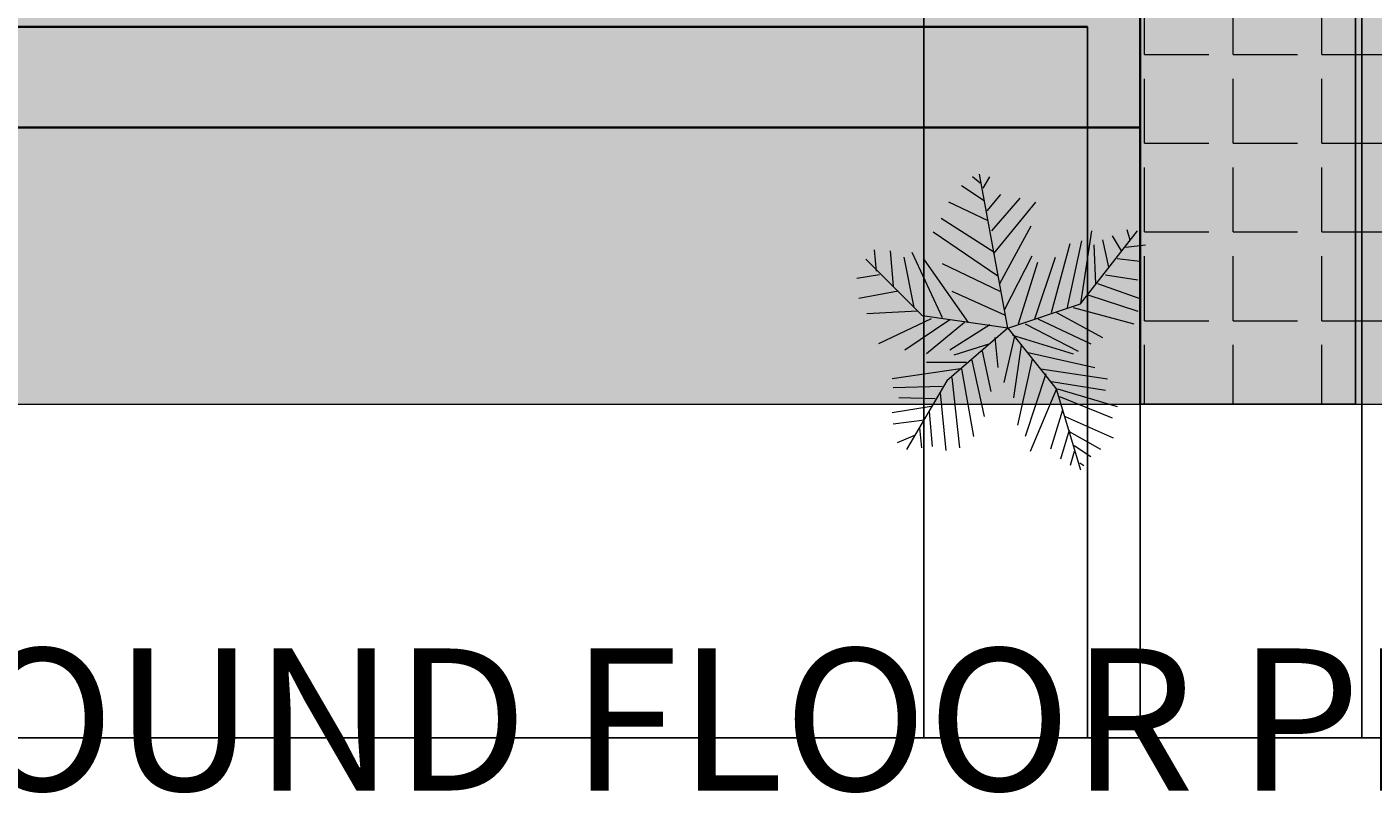
# Model space of a CAD drawing. Units: millimetres. Extents: x 1166 to 16630, y -7192 to 2820.
# Tile 2 of 8: x 2769 to 5842, y -7192 to -5443. Entities that reach past the tile are written whole.
import ezdxf

# ---------------------------------------------------------------- set-up
doc = ezdxf.new("R2010")
doc.units = ezdxf.units.MM
for name, color, linetype, lineweight in [('A-ANNO-DIMS', 2, 'Continuous', 18), ('A-ANNO-TEXT', 7, 'Continuous', 35), ('A-FLOR-PATT', 8, 'Continuous', 13), ('A-WALL', 7, 'Continuous', 35), ('C-SITE-PAVE', 7, 'Continuous', 18), ('L-PLNT', 70, 'Continuous', 18), ('L-PLNT-PATT', 3, 'Continuous', 13)]:
    doc.layers.add(name, color=color, linetype=linetype, lineweight=lineweight)
doc.layers.add('A-FLOR-FNSH-PATT', color=254, linetype='Continuous', lineweight=13, true_color=0xfeeab9)
doc.layers.add('A-WALL-PATT', color=254, linetype='Continuous', lineweight=13, true_color=0xcecce6)
doc.styles.get("Standard").update_dxf_attribs({"font": 'arial.ttf'})
doc.dimstyles.get("Standard").update_dxf_attribs({"dimtxt": 0.18, "dimasz": 0.18, "dimexe": 0.18, "dimexo": 0.0625, "dimgap": 0.09, "dimtad": 0, "dimtih": 1, "dimtoh": 1, "dimdec": 4, "dimzin": 0, "dimdsep": 46, "dimtxsty": 'Standard', "dimcen": 0.09, "dimadec": 0, "dimazin": 0, "dimtfac": 1, "dimtdec": 4, "dimtofl": 0, "dimtmove": 0, "dimatfit": 3, "dimfxl": 1, "dimtolj": 1, "dimtzin": 0, "dimarcsym": 0})

# ---------------------------------------------------------------- blocks, each defined once
blk = doc.blocks.new('*U12')
for p, q in [((-10.186, 53.64), (-13.084, 55.962)), ((0, 0), (-10.5, 57)), ((-9.099, 51.782), (-6.563, 55.962)), ((-8.737, 47.138), (-17.069, 52.711)), ((-7.288, 39.707), (-21.778, 46.673)), ((-7.65, 43.423), (-2.578, 49.46)), ((-5.839, 35.992), (4.667, 48.067)), ((-5.114, 27.632), (10.463, 46.673)), ((-5.114, 28.097), (-24.676, 40.636)), ((-3.665, 19.273), (-27.574, 35.527)), ((-2.941, 16.486), (8.652, 37.85)), ((27, 9), (48, 36)), ((27.127, 9.056), (31.112, 35.992)), ((44.153, 36.456), (45.239, 32.741)), ((16.259, 5.805), (23.142, 31.348)), ((22.055, 7.198), (27.489, 32.277)), ((31.836, 30.883), (32.561, 16.486)), ((35.096, 32.741), (37.27, 22.524)), ((38.719, 34.134), (41.979, 28.561)), ((43.791, 29.954), (51.036, 30.883)), ((-31.5, 4.5), (-52.5, 25.5)), ((-48.585, 21.131), (-49.309, 29.026)), ((-43.513, 28.561), (-42.427, 15.558)), ((-38.442, 26.239), (-34.819, 7.663)), ((-35.544, 28.097), (-24.314, 3.947)), ((-14.533, 2.09), (-30.834, 25.31)), ((-1.129, 6.734), (9.014, 26.704)), ((10.101, 3.483), (17.708, 26.239)), ((40.53, 25.775), (48.862, 24.846)), ((-24.314, 23.917), (-2.941, 13.7)), ((3.942, 1.625), (11.187, 24.381)), ((-47.498, 19.737), (-55.83, 18.344)), ((33.285, 16.486), (48.862, 10.913)), ((36.183, 19.737), (48.137, 17.88)), ((-40.615, 13.7), (-55.105, 10.913)), ((-20.691, 13.7), (-1.129, 4.876)), ((29.662, 12.307), (48.137, 6.269)), ((-33.37, 6.269), (-52.207, 5.34)), ((0, 0), (27, 9)), ((18.07, 5.805), (35.096, -3.483)), ((24.229, 7.663), (46.688, 1.625)), ((-28.299, 3.483), (-47.86, -5.805)), ((-21.416, 3.018), (-38.079, -8.128)), ((0, 0), (-31.5, 4.5)), ((-15.982, 2.09), (-30.11, -9.521)), ((0, 0), (-22.5, -19.5)), ((-6.563, 1.161), (-21.416, -8.128)), ((0, 0), (18, -22.5)), ((6.478, 1.625), (26.04, -8.592)), ((11.187, 3.483), (30.749, -5.805)), ((-4.752, -3.483), (-3.665, -14.629)), ((2.493, -3.019), (-1.491, -20.202)), ((1.769, -2.555), (24.229, -9.521)), ((-6.563, -5.805), (-19.967, -9.985)), ((-9.461, -8.592), (-6.201, -23.453)), ((5.029, -6.27), (2.131, -25.775)), ((7.565, -9.056), (32.198, -14.629)), ((-15.257, -12.772), (-30.11, -12.772)), ((-13.446, -11.378), (-8.737, -32.741)), ((9.014, -11.378), (3.58, -35.992)), ((-17.431, -15.094), (-42.789, -18.809)), ((-22.5, -19.5), (-37.5, -45)), ((-20.691, -18.345), (-17.793, -44.352)), ((-17.069, -15.094), (-12.721, -40.172)), ((14.085, -16.951), (6.478, -40.172)), ((12.274, -15.094), (36.907, -18.809)), ((16.259, -19.738), (36.183, -22.989)), ((-24.314, -21.596), (-42.427, -22.06)), ((-25.038, -23.918), (-22.865, -45.281)), ((18.07, -22.524), (8.289, -45.745)), ((18, -22.5), (27, -52.5)), ((18.433, -22.524), (40.53, -29.026)), ((-28.299, -29.026), (-42.789, -31.348)), ((-26.849, -26.24), (-40.253, -25.775)), ((19.157, -25.311), (38.719, -33.206)), ((-30.834, -34.135), (-42.427, -35.528)), ((-29.023, -30.884), (-27.936, -43.887)), ((20.244, -30.419), (15.897, -44.816)), ((21.331, -32.741), (39.081, -40.636)), ((-34.457, -39.708), (-40.978, -42.494)), ((-32.646, -36.921), (-31.921, -44.352)), ((22.78, -37.85), (19.519, -48.532)), ((22.78, -38.314), (34.372, -44.816)), ((24.591, -43.423), (30.749, -47.603)), ((24.591, -45.745), (23.142, -50.854)), ((26.764, -49.925), (28.213, -50.854))]:
    blk.add_line(p, q)
blk = doc.blocks.new('*D31')
at = {"layer": 'A-ANNO-DIMS', "color": 0, "lineweight": -2, "transparency": 16777216}
for p, q in [((1957, -5450.9), (1957, -7065.6)), ((5189.6, -5442.6), (5189.6, -7065.6)), ((1957.2, -7065.4), (3572.8, -7065.4)), ((5189.4, -7065.4), (3573.8, -7065.4))]:
    blk.add_line(p, q, dxfattribs=at)
at = {"layer": 'A-ANNO-DIMS', "color": 0, "transparency": 16777216}
for points in [[(1957.2, -7065.4), (1957.2, -7065.5), (1957, -7065.4)], [(5189.4, -7065.4), (5189.4, -7065.5), (5189.6, -7065.4)]]:
    blk.add_solid(points, dxfattribs=at)
at = {"layer": 'Defpoints', "color": 0, "transparency": 16777216}
for p in [(1957, -5450.8), (5189.6, -5442.5), (5189.6, -7065.4)]:
    blk.add_point(p, dxfattribs=at)
at = {"layer": 'A-ANNO-DIMS', "color": 0, "transparency": 16777216, "insert": (3573.3, -7065.4), "char_height": 0.18, "attachment_point": 5}
blk.add_mtext('\\A1;3232.6', dxfattribs=at)
blk = doc.blocks.new('*D32')
at = {"layer": 'A-ANNO-DIMS', "color": 0, "lineweight": -2, "transparency": 16777216}
for p, q in [((5309.6, -6304.2), (5309.6, -7065.6)), ((7725.9, -6304.2), (7725.9, -7065.6)), ((5309.8, -7065.4), (6517.3, -7065.4)), ((7725.8, -7065.4), (6518.2, -7065.4))]:
    blk.add_line(p, q, dxfattribs=at)
at = {"layer": 'A-ANNO-DIMS', "color": 0, "transparency": 16777216}
for points in [[(5309.8, -7065.4), (5309.8, -7065.5), (5309.6, -7065.4)], [(7725.8, -7065.4), (7725.8, -7065.5), (7725.9, -7065.4)]]:
    blk.add_solid(points, dxfattribs=at)
at = {"layer": 'Defpoints', "color": 0, "transparency": 16777216}
for p in [(5309.6, -6304.1), (7725.9, -6304.1), (7725.9, -7065.4)]:
    blk.add_point(p, dxfattribs=at)
at = {"layer": 'A-ANNO-DIMS', "color": 0, "transparency": 16777216, "insert": (6517.8, -7065.4), "char_height": 0.18, "attachment_point": 5}
blk.add_mtext('\\A1;2416.3', dxfattribs=at)
blk = doc.blocks.new('*D36')
at = {"layer": 'A-ANNO-DIMS', "color": 0, "lineweight": -2, "transparency": 16777216}
for p, q in [((4815.9, -849.9), (4815.9, -7065.6)), ((5815.9, -849.9), (5815.9, -7065.6)), ((4816.1, -7065.4), (5315.6, -7065.4)), ((5815.8, -7065.4), (5316.3, -7065.4))]:
    blk.add_line(p, q, dxfattribs=at)
at = {"layer": 'A-ANNO-DIMS', "color": 0, "transparency": 16777216}
for points in [[(4816.1, -7065.4), (4816.1, -7065.5), (4815.9, -7065.4)], [(5815.8, -7065.4), (5815.8, -7065.5), (5815.9, -7065.4)]]:
    blk.add_solid(points, dxfattribs=at)
at = {"layer": 'Defpoints', "color": 0, "transparency": 16777216}
for p in [(4815.9, -849.8), (5815.9, -849.8), (5815.9, -7065.4)]:
    blk.add_point(p, dxfattribs=at)
at = {"layer": 'A-ANNO-DIMS', "color": 0, "transparency": 16777216, "insert": (5315.9, -7065.4), "char_height": 0.18, "attachment_point": 5}
blk.add_mtext('\\A1;1000', dxfattribs=at)
blk = doc.blocks.new('*D39')
at = {"layer": 'A-ANNO-DIMS', "color": 0, "lineweight": -2, "transparency": 16777216}
for p, q in [((5309.7, -2642.5), (5801.8, -2642.5)), ((5801.6, -2642.7), (5801.6, -4473.2)), ((5801.6, -6304), (5801.6, -4473.5)), ((5309.7, -6304.1), (5801.8, -6304.1))]:
    blk.add_line(p, q, dxfattribs=at)
at = {"layer": 'A-ANNO-DIMS', "color": 0, "transparency": 16777216}
for points in [[(5801.6, -2642.7), (5801.6, -2642.7), (5801.6, -2642.5)], [(5801.6, -6304), (5801.6, -6304), (5801.6, -6304.1)]]:
    blk.add_solid(points, dxfattribs=at)
at = {"layer": 'Defpoints', "color": 0, "transparency": 16777216}
for p in [(5309.6, -2642.5), (5309.6, -6304.1), (5801.6, -6304.1)]:
    blk.add_point(p, dxfattribs=at)
at = {"layer": 'A-ANNO-DIMS', "color": 0, "transparency": 16777216, "insert": (5801.6, -4473.3), "char_height": 0.18, "attachment_point": 5}
blk.add_mtext('\\A1;3661.6', dxfattribs=at)

msp = doc.modelspace()

# ---------------------------------------------------------------- hatches: boundary and pattern name
at = {"layer": 'A-FLOR-FNSH-PATT', "transparency": 33554523}
h = msp.add_hatch(color=256, dxfattribs=at)
h.dxf.hatch_style = 1
h.paths.add_polyline_path([(7725.939, 2327.462), (1725.939, 2327.462), (1725.939, -5672.538), (5309.615, -5672.538), (5309.615, -2642.538), (5189.615, -2642.538), (5189.615, -5442.538), (1955.939, -5442.538), (1955.939, 2097.462), (4665.939, 2097.462), (4665.939, 150.2), (4815.939, 150.2, -0.40145271), (5814.982, -806.05), (5815.939, -806.05), (5815.939, -849.8), (4815.939, -849.8), (4785.939, -849.8), (4785.939, -902.538), (7495.939, -902.538), (7495.939, -2522.538), (4884.014, -2522.538), (4884.014, -2642.538), (7725.939, -2642.538)], flags=17)
h.paths.add_polyline_path([(6066.077, 618.421), (6066.077, 1624.186), (7407.098, 1624.186), (7407.098, 618.421)], flags=16)
h.paths.add_polyline_path([(4979.212, 660.219), (4799.278, 660.219), (4799.278, 780.174), (4789.282, 790.171), (4789.282, 870.141), (4799.278, 880.137), (4799.278, 1259.997), (4979.212, 1259.997), (4979.212, 1230.008), (4989.208, 1230.008), (4989.208, 1110.052), (4979.212, 1110.052), (4979.212, 1100.056), (4989.208, 1100.056), (4989.208, 980.1), (4979.212, 980.1), (4979.212, 950.111), (4989.208, 950.111), (4989.208, 940.115, -0.09090909), (4989.208, 720.196), (4989.208, 710.2), (4979.212, 710.2)], flags=16)
h.paths.add_polyline_path([(4974.214, 665.217), (4804.276, 665.217), (4804.276, 1254.999), (4974.214, 1254.999)], flags=0)
h.paths.add_polyline_path([(6910.92, 618.421), (6910.92, 873.215), (7165.714, 873.215), (7165.714, 1490.084), (7386.983, 1490.084), (7386.983, 1141.419), (7165.714, 1141.419), (7165.714, 1101.188), (7386.983, 1101.188), (7386.983, 752.523), (7132.189, 752.523), (7132.189, 839.689)], flags=16)
h.paths.add_polyline_path([(4815.939, 150.2), (4665.939, 150.2), (4665.939, 1500.697), (2460.545, 1500.697), (2460.545, -402.538), (3575.939, -402.538), (3575.939, -1706.64), (3463.439, -1706.64, 0.40145271), (2714.158, -2423.828), (3463.439, -2423.828), (3463.439, -2456.64), (3455.939, -2522.538), (3455.939, -2456.64), (2713.439, -2456.64), (2713.439, -2423.828), (2714.158, -2423.828, -0.39855266), (3455.939, -1706.678), (3455.939, -1706.64), (3575.939, -1706.64), (3575.939, -402.538), (2460.545, -402.538), (2460.545, 1500.697), (4665.939, 1500.697), (4665.939, 150.2), (4785.939, 150.2), (4785.939, 2097.462), (7495.939, 2097.462), (7495.939, -2522.538), (4884.014, -2522.538), (4884.014, -2642.538), (7725.939, -2642.538), (7725.939, 2327.462), (1725.939, 2327.462), (1725.939, -5672.538), (5309.615, -5672.538), (5309.615, -2642.538), (4884.014, -2642.538), (4884.014, -2522.538), (4884.014, -1822.538), (4665.939, -1822.538), (4665.939, -1722.538), (4665.939, -1022.538), (4665.939, -849.8), (4815.939, -849.8), (4815.939, -806.05), (5814.982, -806.05, 0.40145271)])
h.paths.add_polyline_path([(1955.939, -4323.626), (1965.936, -4313.63), (1965.936, -3933.77), (2145.869, -3933.77), (2145.869, -3963.759), (2155.866, -3963.759), (2155.866, -4083.715), (2145.869, -4083.715), (2145.869, -4093.711), (2155.866, -4093.711), (2155.866, -4213.667), (2145.869, -4213.667), (2145.869, -4243.656), (2155.866, -4243.656), (2155.866, -4253.652, -0.09090909), (2155.866, -4473.571), (2155.866, -4483.567), (2145.869, -4483.567), (2145.869, -4533.549), (1965.936, -4533.549), (1965.936, -4413.593), (1955.939, -4403.597)], flags=16)
h.paths.add_polyline_path([(3017.672, -1268.685), (3017.672, -1558.932), (2092.538, -1558.932), (2092.538, -1268.685)], flags=16)
h.paths.add_polyline_path([(2768.799, -687.028), (2664.904, -687.028), (2696.871, -782.93, -0.50132349), (2617.667, -1084.405, -0.13289091), (2584.271, -1084.405, -0.50131678), (2505.065, -782.933), (2537.033, -687.028), (2489.082, -687.028), (2489.082, -711.004), (2441.13, -711.004), (2441.13, -687.028), (2433.138, -687.028), (2433.138, -559.158), (2768.799, -559.158)], flags=16)
h.paths.add_polyline_path([(2752.815, -655.061, -0.41421356), (2740.827, -671.045), (2465.106, -671.045, -0.41421356), (2449.122, -659.057), (2449.122, -591.126, -0.41421356), (2461.11, -575.142), (2736.831, -575.142, -0.41421356), (2752.815, -587.13)], flags=0)
h.paths.add_polyline_path([(2627.247, -1063.016, -0.21500378), (2574.691, -1063.016, -0.48007965), (2537.034, -782.931), (2664.904, -782.931, -0.4800795)], flags=0)
h.paths.add_polyline_path([(4505.634, -3647.875), (4977.863, -3647.875, -0.19047621), (4977.864, -5173.541), (4505.634, -5173.541), (4505.634, -5064.565), (4533.929, -5064.565), (4533.929, -3756.851), (4505.634, -3756.851)], flags=16)
h.paths.add_polyline_path([(4880.114, -4192.756), (5003.372, -4192.756, -0.04962821), (5003.372, -4628.66), (4880.114, -4628.66)], flags=0)
h.paths.add_polyline_path([(2140.871, -3938.769), (2140.871, -4528.551), (1970.934, -4528.551), (1970.934, -3938.769)], flags=0)
h.paths.add_polyline_path([(7495.939, -1022.538), (6660.699, -1022.538), (6660.699, -1722.538, -0.21291191), (6697.901, -1739.132)], flags=16)
h.paths.add_polyline_path([(7495.939, -1022.538), (6697.901, -1739.132, -0.18498743), (6710.699, -1772.538), (7495.939, -1772.538)], flags=16)
h.paths.add_polyline_path([(7495.939, -1772.538), (6710.699, -1772.538, -0.18498743), (6697.901, -1805.944), (7495.939, -2522.538)], flags=16)
h.paths.add_polyline_path([(6697.901, -1805.944, -0.21291191), (6660.699, -1822.538), (6660.699, -2522.538), (7495.939, -2522.538)], flags=16)
h.paths.add_polyline_path([(6660.699, -1822.538), (6438.613, -1822.538), (6438.613, -2522.538), (6660.699, -2522.538)], flags=16)
h.paths.add_polyline_path([(6438.613, -1822.538), (6216.528, -1822.538), (6216.528, -2522.538), (6438.613, -2522.538)], flags=16)
h.paths.add_polyline_path([(6216.528, -1822.538), (5994.442, -1822.538), (5994.442, -2522.538), (6216.528, -2522.538)], flags=16)
h.paths.add_polyline_path([(5994.442, -1822.538), (5772.357, -1822.538), (5772.357, -2522.538), (5994.442, -2522.538)], flags=16)
h.paths.add_polyline_path([(5550.271, -1822.538), (5328.185, -1822.538), (5328.185, -2522.538), (5550.271, -2522.538)], flags=16)
h.paths.add_polyline_path([(5328.185, -1822.538), (5106.1, -1822.538), (5106.1, -2522.538), (5328.185, -2522.538)], flags=16)
h.paths.add_polyline_path([(5106.1, -1822.538), (4884.014, -1822.538), (4884.014, -2522.538), (5106.1, -2522.538)], flags=16)
h.paths.add_polyline_path([(4884.014, -1022.538), (4665.939, -1022.538), (4665.939, -1722.538), (4884.014, -1722.538)], flags=16)
h.paths.add_polyline_path([(5106.1, -1022.538), (4884.014, -1022.538), (4884.014, -1722.538), (5106.1, -1722.538)], flags=16)
h.paths.add_polyline_path([(5550.271, -1022.538), (5328.185, -1022.538), (5328.185, -1722.538), (5550.271, -1722.538)], flags=16)
h.paths.add_polyline_path([(5328.185, -1022.538), (5106.1, -1022.538), (5106.1, -1722.538), (5328.185, -1722.538)], flags=16)
h.paths.add_polyline_path([(5772.357, -1022.538), (5550.271, -1022.538), (5550.271, -1722.538), (5772.357, -1722.538)], flags=16)
h.paths.add_polyline_path([(5994.442, -1022.538), (5772.357, -1022.538), (5772.357, -1722.538), (5994.442, -1722.538)], flags=16)
h.paths.add_polyline_path([(6216.528, -1022.538), (5994.442, -1022.538), (5994.442, -1722.538), (6216.528, -1722.538)], flags=16)
h.paths.add_polyline_path([(6660.699, -1022.538), (6438.613, -1022.538), (6438.613, -1722.538), (6660.699, -1722.538)], flags=16)
h.paths.add_polyline_path([(6438.613, -1022.538), (6216.528, -1022.538), (6216.528, -1722.538), (6438.613, -1722.538)], flags=16)
h.paths.add_polyline_path([(5772.357, -1822.538), (5550.271, -1822.538), (5550.271, -2522.538), (5772.357, -2522.538)], flags=16)
h.paths.add_polyline_path([(6660.699, -1722.538), (6438.613, -1722.538), (4665.939, -1722.538), (4665.939, -1822.538), (6660.699, -1822.538, 0.21291191), (6697.901, -1805.944, 0.64892437)], flags=16)
h.paths.add_polyline_path([(5860.25, -44.006), (7154.504, -44.006), (7154.504, 215.689), (5860.25, 215.689)], flags=24)
h.paths.add_polyline_path([(2102.336, -1543.656), (3007.075, -1543.656), (3007.075, -1283.961), (2102.336, -1283.961)], flags=8)
h.paths.add_polyline_path([(2887.503, -4248.68), (3740.372, -4248.68), (3740.372, -3989.156), (2887.503, -3989.156)], flags=24)
h.paths.add_polyline_path([(2999.436, 433.054), (4111.829, 433.054), (4111.829, 692.578), (2999.436, 692.578)], flags=24)
at = {"layer": 'A-FLOR-FNSH-PATT', "transparency": 33554590}
h = msp.add_hatch(color=256, dxfattribs=at)
h.dxf.hatch_style = 1
h.paths.add_polyline_path([(5309.615, -2642.538), (5309.615, -6304.141), (7725.939, -6304.141), (7725.939, -5672.538), (7725.939, -2642.538)])
edge = h.paths.add_edge_path(flags=16)
edge.add_ellipse((-448.972, -3645.43), major_axis=(-7430.723, 0), ratio=0.84230387, start_angle=182.1799503, end_angle=183.6504276, ccw=False)
edge.add_line((6974.174, -3362.862), (6984.716, -3362.862))
edge.add_ellipse((6982.281, -3380.397), major_axis=(-20.817, 0), ratio=0.84230387, start_angle=180, end_angle=270, ccw=False)
edge.add_line((7003.098, -3380.397), (7003.098, -3722.916))
edge.add_ellipse((6982.281, -3720.865), major_axis=(20.817, 0), ratio=0.84230387, start_angle=270, end_angle=360, ccw=False)
edge.add_ellipse((-142030.923, -3973.064), major_axis=(149013.204, 0), ratio=0.8423038695, start_angle=-0.38386678, end_angle=0.09022909, ccw=False)
edge.add_line((6977.567, -4971.397), (6984.47, -4971.397))
edge.add_ellipse((6982.281, -4988.932), major_axis=(20.817, 0), ratio=0.84230387, start_angle=0, end_angle=90, ccw=False)
edge.add_line((7003.098, -4988.932), (7003.098, -5331.243))
edge.add_ellipse((6982.281, -5329.4), major_axis=(-20.817, 0), ratio=0.84230387, start_angle=90, end_angle=180, ccw=False)
edge.add_line((6982.281, -5346.934), (6973.354, -5346.934))
edge.add_ellipse((-142030.923, -3973.064), major_axis=(149013.204, 0), ratio=0.8423038695, start_angle=-0.6186432, end_angle=-0.52827147, ccw=False)
edge.add_ellipse((6960.189, -5606.903), major_axis=(-31.226, 0), ratio=0.84230387, start_angle=179.371763, end_angle=248.464757, ccw=False)
edge.add_ellipse((-142041.332, -3973.064), major_axis=(-149045.372, 0), ratio=0.8423038661, start_angle=179.35344592, end_angle=179.3717628, ccw=False)
edge.add_ellipse((6916.87, -5654.054), major_axis=(-73.802, 0), ratio=0.84230387, start_angle=90, end_angle=179.353446, ccw=False)
edge.add_line((6916.87, -5716.218), (5995.23, -5716.218))
edge.add_ellipse((5995.23, -5654.054), major_axis=(73.802, 0), ratio=0.84230387, start_angle=180.646554, end_angle=270, ccw=False)
edge.add_ellipse((154953.432, -3973.064), major_axis=(-149045.372, 0), ratio=0.8423038697, start_angle=0.62823722, end_angle=0.6465541, ccw=False)
edge.add_ellipse((5951.911, -5606.903), major_axis=(31.226, 0), ratio=0.84230387, start_angle=111.535244, end_angle=180.628237, ccw=False)
edge.add_ellipse((154943.023, -3973.064), major_axis=(-149013.204, 0), ratio=0.8423038695, start_angle=0.52827147, end_angle=0.6465541, ccw=False)
edge.add_line((5938.746, -5346.934), (5927.384, -5346.934))
edge.add_ellipse((5929.819, -5329.4), major_axis=(20.817, 0), ratio=0.84230387, start_angle=180, end_angle=270, ccw=False)
edge.add_line((5909.002, -5329.4), (5909.002, -4986.881))
edge.add_ellipse((5929.819, -4988.932), major_axis=(-20.817, 0), ratio=0.84230387, start_angle=-90, end_angle=0, ccw=False)
edge.add_line((5929.819, -4971.397), (5934.533, -4971.397))
edge.add_ellipse((154943.023, -3973.064), major_axis=(-149013.204, 0), ratio=0.8423038695, start_angle=-0.09022909, end_angle=0.38386678, ccw=False)
edge.add_ellipse((5929.819, -3720.865), major_axis=(-20.817, 0), ratio=0.84230387, start_angle=0, end_angle=90, ccw=False)
edge.add_line((5909.002, -3720.865), (5909.002, -3378.346))
edge.add_ellipse((5929.819, -3380.397), major_axis=(20.817, 0), ratio=0.84230387, start_angle=90, end_angle=180, ccw=False)
edge.add_line((5929.819, -3362.862), (5937.926, -3362.862))
edge.add_ellipse((13361.072, -3645.43), major_axis=(7430.723, 0), ratio=0.84230387, start_angle=176.3495724, end_angle=177.8200497, ccw=False)
edge.add_ellipse((6843.239, -6808.261), major_axis=(4407.333, 0), ratio=0.84230387, start_angle=102.125966, end_angle=103.780529, ccw=False)
edge.add_ellipse((6843.239, -6711.831), major_axis=(4294.728, 0), ratio=0.84230387, start_angle=100.209539, end_angle=102.444627, ccw=False)
edge.add_ellipse((5718.978, -189.342), major_axis=(-3530.283, 0), ratio=0.84230387, start_angle=99.256566, end_angle=102.554933)
edge.add_line((6369.843, -3111.939), (6452.047, -3066.483))
edge.add_ellipse((6456.05, -3074.757), major_axis=(-10.409, 0), ratio=0.84230387, start_angle=270, end_angle=307.93313, ccw=False)
edge.add_ellipse((6456.05, -3074.757), major_axis=(-10.409, 0), ratio=0.84230387, start_angle=232.06687, end_angle=270, ccw=False)
edge.add_line((6461.762, -3067.428), (6542.257, -3111.939))
edge.add_ellipse((7193.122, -189.342), major_axis=(3530.283, 0), ratio=0.84230387, start_angle=257.445067, end_angle=260.743434)
edge.add_ellipse((6068.861, -6711.831), major_axis=(4294.728, 0), ratio=0.84230387, start_angle=77.555373, end_angle=79.790461, ccw=False)
edge.add_ellipse((6068.861, -6808.261), major_axis=(-4407.333, 0), ratio=0.84230387, start_angle=256.219471, end_angle=257.874034, ccw=False)
edge = h.paths.add_edge_path(flags=0)
edge.add_ellipse((5799.636, -3484.806), major_axis=(790.133, 0), ratio=0.84230387, start_angle=0, end_angle=29.43857, ccw=False)
edge.add_line((6589.77, -3484.806), (6589.77, -3517.866))
edge.add_line((6589.77, -3517.866), (6615.397, -3517.866))
edge.add_ellipse((6612.95, -3526.633), major_axis=(10.409, 0), ratio=0.84230387, start_angle=45.519789, end_angle=90, ccw=False)
edge.add_line((6619.584, -3519.877), (6697.577, -3574.216))
edge.add_line((6697.577, -3574.216), (6697.577, -3782.552))
edge.add_ellipse((6643.673, -3780.461), major_axis=(5.016, 89.187), ratio=0.60383358, start_angle=106.342592, end_angle=270.997986, ccw=False)
edge.add_line((6589.77, -3793.028), (6589.77, -3484.806))
edge.add_ellipse((5799.636, -3484.806), major_axis=(790.133, 0), ratio=0.84230387, start_angle=0, end_angle=29.43857)
edge.add_ellipse((7112.464, -3484.806), major_axis=(-790.133, 0), ratio=0.84230387, start_angle=-29.43857, end_angle=0)
edge.add_line((6322.33, -3484.806), (6322.33, -3793.028))
edge.add_ellipse((6268.427, -3780.461), major_axis=(-5.016, 89.187), ratio=0.60383358, start_angle=89.002014, end_angle=253.657408, ccw=False)
edge.add_line((6214.523, -3782.552), (6214.523, -3574.216))
edge.add_line((6214.523, -3574.216), (6294.401, -3518.564))
edge.add_ellipse((6299.15, -3526.633), major_axis=(10.409, 0), ratio=0.84230387, start_angle=90, end_angle=134.480211, ccw=False)
edge.add_line((6299.15, -3517.866), (6322.33, -3517.866))
edge.add_line((6322.33, -3517.866), (6322.33, -3484.806))
edge.add_ellipse((7112.464, -3484.806), major_axis=(-790.133, 0), ratio=0.84230387, start_angle=-29.43857, end_angle=0, ccw=False)
edge = h.paths.add_edge_path(flags=0)
edge.add_line((6899.672, -4051.113), (6868.937, -4281.474))
edge.add_ellipse((6495.43, -5170.363), major_axis=(1119.455, 0), ratio=0.84230387, start_angle=67.208085, end_angle=85.12993)
edge.add_line((6575.565, -4229.86), (6336.535, -4229.86))
edge.add_ellipse((6416.67, -5170.363), major_axis=(1119.455, 0), ratio=0.84230387, start_angle=94.87007, end_angle=112.791915)
edge.add_line((6043.163, -4281.474), (6012.428, -4051.113))
edge.add_ellipse((6380.264, -4969.144), major_axis=(1150.303, 0), ratio=0.84230387, start_angle=94.277421, end_angle=111.834954, ccw=False)
edge.add_line((6307.939, -4002.156), (6604.161, -4002.156))
edge.add_ellipse((6531.836, -4969.144), major_axis=(-1150.303, 0), ratio=0.84230387, start_angle=248.165046, end_angle=265.722579, ccw=False)
edge = h.paths.add_edge_path(flags=0)
edge.add_ellipse((-142030.923, -3973.064), major_axis=(-148992.387, 0), ratio=0.8423038695, start_angle=179.62223581, end_angle=179.94440569, ccw=False)
edge.add_line((6956.9, -4955.389), (6903.068, -4744.03))
edge.add_ellipse((-45118.924, -4413.46), major_axis=(52023.473, 0), ratio=0.84230387, start_angle=-0.3640763, end_angle=0.1208974)
edge.add_line((6904.386, -4303.688), (6961.365, -4117.632))
edge = h.paths.add_edge_path(flags=0)
edge.add_line((5950.735, -4117.632), (6007.714, -4303.688))
edge.add_ellipse((58031.024, -4413.46), major_axis=(-52023.473, 0), ratio=0.84230387, start_angle=-0.1208974, end_angle=0.3640763)
edge.add_line((6009.031, -4744.03), (5955.2, -4955.389))
edge.add_ellipse((154943.023, -3973.064), major_axis=(-148992.387, 0), ratio=0.8423038696, start_angle=0.05559431, end_angle=0.37776419, ccw=False)
edge = h.paths.add_edge_path(flags=0)
edge.add_line((6868.937, -5013.198), (6868.937, -5277.993))
edge.add_ellipse((6456.05, -3571.079), major_axis=(2068.116, 0), ratio=0.84230387, start_angle=256.401865, end_angle=283.598135, ccw=False)
edge.add_line((6043.163, -5277.993), (6043.163, -5013.198))
edge.add_ellipse((6456.05, -3306.285), major_axis=(2068.116, 0), ratio=0.84230387, start_angle=256.401865, end_angle=283.598135)
edge = h.paths.add_edge_path(flags=0)
edge.add_ellipse((6827.303, -5415.313), major_axis=(-41.634, 0), ratio=0.84230387, start_angle=180, end_angle=270, ccw=False)
edge.add_line((6868.937, -5415.313), (6868.937, -5689.123))
edge.add_line((6868.937, -5689.123), (6043.163, -5689.123))
edge.add_line((6043.163, -5689.123), (6043.163, -5415.313))
edge.add_ellipse((6084.797, -5415.313), major_axis=(-41.634, 0), ratio=0.84230387, start_angle=-90, end_angle=0, ccw=False)
edge.add_line((6084.797, -5380.245), (6827.303, -5380.245))
h.paths.add_polyline_path([(3455.939, -522.538), (1955.939, -522.538), (1955.939, -2522.538), (3455.939, -2522.538), (3455.939, -2456.64), (2713.439, -2456.64), (2713.439, -2423.828), (2714.158, -2423.828, -0.39855266), (3455.939, -1706.678)])
h.paths.add_polyline_path([(2617.667, -1084.405, -0.13289091), (2584.271, -1084.405, -0.50131678), (2505.065, -782.933), (2537.033, -687.028), (2489.082, -687.028), (2489.082, -711.004), (2441.13, -711.004), (2441.13, -695.02), (2473.098, -695.02), (2473.098, -687.028), (2433.138, -687.028), (2433.138, -559.158), (2768.799, -559.158), (2768.799, -687.028), (2664.904, -687.028), (2696.871, -782.93, -0.50132349)], flags=16)
h.paths.add_polyline_path([(2627.247, -1063.016, -0.21500378), (2574.691, -1063.016, -0.48007965), (2537.034, -782.931), (2664.904, -782.931, -0.4800795)], flags=0)
h.paths.add_polyline_path([(2736.831, -671.045), (2465.106, -671.045, -0.50000012), (2449.122, -655.061), (2449.122, -591.126, -0.50000012), (2465.106, -575.142), (2736.831, -575.142, -0.50000012), (2752.815, -591.126), (2752.815, -655.061, -0.50000012)], flags=0)
h.paths.add_polyline_path([(5931.782, -6111.826), (7070.31, -6111.826), (7070.31, -5852.302), (5931.782, -5852.302)], flags=24)
h.paths.add_polyline_path([(2102.336, -1543.656), (3007.075, -1543.656), (3007.075, -1283.961), (2102.336, -1283.961)], flags=24)
at = {"layer": 'A-FLOR-PATT', "transparency": 33554564}
h = msp.add_hatch(dxfattribs=at)
h.set_pattern_fill('ANGLE', color=256, scale=29)
h.set_pattern_definition([(0, (-8657.52, -11987.85), (0, 202.565), [147.32, -55.245]), (90, (-8657.52, -11987.85), (-202.565, 1e-14), [147.32, -55.245])])
h.paths.add_polyline_path([(7725.939, -2642.538), (5309.615, -2642.538), (5309.615, -6304.141), (7725.939, -6304.141), (7725.939, -5672.538)])
edge = h.paths.add_edge_path(flags=16)
edge.add_ellipse((-142030.923, -3973.064), major_axis=(149013.204, 0), ratio=0.8423038695, start_angle=-0.38386678, end_angle=0.09022909, ccw=False)
edge.add_ellipse((6982.281, -4988.932), major_axis=(20.817, 0), ratio=0.84230387, start_angle=0, end_angle=90, ccw=False)
edge.add_line((7003.098, -4988.932), (7003.098, -5329.4))
edge.add_ellipse((6982.281, -5329.4), major_axis=(-20.817, 0), ratio=0.84230387, start_angle=90, end_angle=180, ccw=False)
edge.add_line((6982.281, -5346.934), (6973.354, -5346.934))
edge.add_ellipse((-142030.923, -3973.064), major_axis=(149013.204, 0), ratio=0.8423038695, start_angle=-0.6186432, end_angle=-0.52827147, ccw=False)
edge.add_ellipse((6960.189, -5606.903), major_axis=(-31.226, 0), ratio=0.84230387, start_angle=179.371763, end_angle=248.464757, ccw=False)
edge.add_ellipse((-142041.332, -3973.064), major_axis=(-149045.372, 0), ratio=0.8423038661, start_angle=179.35344592, end_angle=179.3717628, ccw=False)
edge.add_ellipse((6916.87, -5654.054), major_axis=(-73.802, 0), ratio=0.84230387, start_angle=90, end_angle=179.353446, ccw=False)
edge.add_line((6916.87, -5716.218), (5995.23, -5716.218))
edge.add_ellipse((5995.23, -5654.054), major_axis=(73.802, 0), ratio=0.84230387, start_angle=180.646554, end_angle=270, ccw=False)
edge.add_ellipse((154953.432, -3973.064), major_axis=(-149045.372, 0), ratio=0.8423038697, start_angle=0.62823722, end_angle=0.6465541, ccw=False)
edge.add_ellipse((5951.911, -5606.903), major_axis=(31.226, 0), ratio=0.84230387, start_angle=111.535244, end_angle=180.628237, ccw=False)
edge.add_ellipse((154943.023, -3973.064), major_axis=(-149013.204, 0), ratio=0.8423038695, start_angle=0.52827147, end_angle=0.6465541, ccw=False)
edge.add_line((5938.746, -5346.934), (5929.819, -5346.934))
edge.add_ellipse((5929.819, -5329.4), major_axis=(20.817, 0), ratio=0.84230387, start_angle=180, end_angle=270, ccw=False)
edge.add_line((5909.002, -5329.4), (5909.002, -4988.932))
edge.add_ellipse((5929.819, -4988.932), major_axis=(-20.817, 0), ratio=0.84230387, start_angle=-90, end_angle=0, ccw=False)
edge.add_ellipse((154943.023, -3973.064), major_axis=(-149013.204, 0), ratio=0.8423038695, start_angle=-0.09022909, end_angle=0.38386678, ccw=False)
edge.add_ellipse((5929.819, -3720.865), major_axis=(-20.817, 0), ratio=0.84230387, start_angle=0, end_angle=90, ccw=False)
edge.add_line((5909.002, -3720.865), (5909.002, -3380.397))
edge.add_ellipse((5929.819, -3380.397), major_axis=(20.817, 0), ratio=0.84230387, start_angle=90, end_angle=180, ccw=False)
edge.add_line((5929.819, -3362.862), (5937.926, -3362.862))
edge.add_ellipse((13361.072, -3645.43), major_axis=(7430.723, 0), ratio=0.84230387, start_angle=176.3495724, end_angle=177.8200497, ccw=False)
edge.add_ellipse((6843.239, -6808.261), major_axis=(4407.333, 0), ratio=0.84230387, start_angle=102.125966, end_angle=103.780529, ccw=False)
edge.add_ellipse((6843.239, -6711.831), major_axis=(4294.728, 0), ratio=0.84230387, start_angle=100.209539, end_angle=102.444627, ccw=False)
edge.add_ellipse((5718.978, -189.342), major_axis=(-3530.283, 0), ratio=0.84230387, start_angle=99.256566, end_angle=102.554933)
edge.add_line((6369.843, -3111.939), (6453.506, -3065.676))
edge.add_ellipse((6456.05, -3074.757), major_axis=(-10.409, 0), ratio=0.84230387, start_angle=232.06687, end_angle=270, ccw=False)
edge.add_line((6460.053, -3066.483), (6542.257, -3111.939))
edge.add_ellipse((7193.122, -189.342), major_axis=(3530.283, 0), ratio=0.84230387, start_angle=257.445067, end_angle=260.743434)
edge.add_ellipse((6068.861, -6711.831), major_axis=(4294.728, 0), ratio=0.84230387, start_angle=77.555373, end_angle=79.790461, ccw=False)
edge.add_ellipse((6068.861, -6808.261), major_axis=(-4407.333, 0), ratio=0.84230387, start_angle=256.219471, end_angle=257.874034, ccw=False)
edge.add_ellipse((-448.972, -3645.43), major_axis=(-7430.723, 0), ratio=0.84230387, start_angle=182.1799503, end_angle=183.6504276, ccw=False)
edge.add_line((6974.174, -3362.862), (6982.281, -3362.862))
edge.add_ellipse((6982.281, -3380.397), major_axis=(-20.817, 0), ratio=0.84230387, start_angle=180, end_angle=270, ccw=False)
edge.add_line((7003.098, -3380.397), (7003.098, -3720.865))
edge.add_ellipse((6982.281, -3720.865), major_axis=(20.817, 0), ratio=0.84230387, start_angle=270, end_angle=360, ccw=False)
edge = h.paths.add_edge_path(flags=0)
edge.add_ellipse((-142030.923, -3973.064), major_axis=(-148992.387, 0), ratio=0.8423038695, start_angle=179.62223581, end_angle=179.94440569, ccw=False)
edge.add_line((6956.9, -4955.389), (6903.068, -4744.03))
edge.add_ellipse((-45118.924, -4413.46), major_axis=(52023.473, 0), ratio=0.84230387, start_angle=-0.3640763, end_angle=0.1208974)
edge.add_line((6904.386, -4303.688), (6961.365, -4117.632))
edge = h.paths.add_edge_path(flags=0)
edge.add_line((6899.672, -4051.113), (6868.937, -4281.474))
edge.add_ellipse((6495.43, -5170.363), major_axis=(1119.455, 0), ratio=0.84230387, start_angle=67.208085, end_angle=85.12993)
edge.add_line((6575.565, -4229.86), (6336.535, -4229.86))
edge.add_ellipse((6416.67, -5170.363), major_axis=(1119.455, 0), ratio=0.84230387, start_angle=94.87007, end_angle=112.791915)
edge.add_line((6043.163, -4281.474), (6012.428, -4051.113))
edge.add_ellipse((6380.264, -4969.144), major_axis=(1150.303, 0), ratio=0.84230387, start_angle=94.277421, end_angle=111.834954, ccw=False)
edge.add_line((6307.939, -4002.156), (6604.161, -4002.156))
edge.add_ellipse((6531.836, -4969.144), major_axis=(-1150.303, 0), ratio=0.84230387, start_angle=248.165046, end_angle=265.722579, ccw=False)
edge = h.paths.add_edge_path(flags=0)
edge.add_ellipse((6643.673, -3780.461), major_axis=(5.016, 89.187), ratio=0.60383358, start_angle=106.342592, end_angle=270.997986, ccw=False)
edge.add_line((6589.77, -3793.028), (6589.77, -3484.806))
edge.add_ellipse((5799.636, -3484.806), major_axis=(790.133, 0), ratio=0.84230387, start_angle=0, end_angle=29.43857)
edge.add_ellipse((7112.464, -3484.806), major_axis=(-790.133, 0), ratio=0.84230387, start_angle=-29.43857, end_angle=0)
edge.add_line((6322.33, -3484.806), (6322.33, -3793.028))
edge.add_ellipse((6268.427, -3780.461), major_axis=(-5.016, 89.187), ratio=0.60383358, start_angle=89.002014, end_angle=253.657408, ccw=False)
edge.add_line((6214.523, -3782.552), (6214.523, -3574.216))
edge.add_line((6214.523, -3574.216), (6295.403, -3517.866))
edge.add_line((6295.403, -3517.866), (6322.33, -3517.866))
edge.add_line((6322.33, -3517.866), (6322.33, -3484.806))
edge.add_ellipse((7112.464, -3484.806), major_axis=(-790.133, 0), ratio=0.84230387, start_angle=-29.43857, end_angle=0, ccw=False)
edge.add_ellipse((5799.636, -3484.806), major_axis=(790.133, 0), ratio=0.84230387, start_angle=0, end_angle=29.43857, ccw=False)
edge.add_line((6589.77, -3484.806), (6589.77, -3517.866))
edge.add_line((6589.77, -3517.866), (6616.697, -3517.866))
edge.add_line((6616.697, -3517.866), (6697.577, -3574.216))
edge.add_line((6697.577, -3574.216), (6697.577, -3782.552))
edge = h.paths.add_edge_path(flags=0)
edge.add_line((6868.937, -5013.198), (6868.937, -5277.993))
edge.add_ellipse((6456.05, -3571.079), major_axis=(2068.116, 0), ratio=0.84230387, start_angle=256.401865, end_angle=283.598135, ccw=False)
edge.add_line((6043.163, -5277.993), (6043.163, -5013.198))
edge.add_ellipse((6456.05, -3306.285), major_axis=(2068.116, 0), ratio=0.84230387, start_angle=256.401865, end_angle=283.598135)
edge = h.paths.add_edge_path(flags=0)
edge.add_ellipse((58031.024, -4413.46), major_axis=(-52023.473, 0), ratio=0.84230387, start_angle=-0.1208974, end_angle=0.3640763)
edge.add_line((6009.031, -4744.03), (5955.2, -4955.389))
edge.add_ellipse((154943.023, -3973.064), major_axis=(-148992.387, 0), ratio=0.8423038696, start_angle=0.05559431, end_angle=0.37776419, ccw=False)
edge.add_line((5950.735, -4117.632), (6007.714, -4303.688))
edge = h.paths.add_edge_path(flags=0)
edge.add_ellipse((6827.303, -5415.313), major_axis=(-41.634, 0), ratio=0.84230387, start_angle=180, end_angle=270, ccw=False)
edge.add_line((6868.937, -5415.313), (6868.937, -5689.123))
edge.add_line((6868.937, -5689.123), (6043.163, -5689.123))
edge.add_line((6043.163, -5689.123), (6043.163, -5415.313))
edge.add_ellipse((6084.797, -5415.313), major_axis=(-41.634, 0), ratio=0.84230387, start_angle=-90, end_angle=0, ccw=False)
edge.add_line((6084.797, -5380.245), (6827.303, -5380.245))
at = {"layer": 'A-WALL-PATT'}
h = msp.add_hatch(color=256, dxfattribs=at)
h.dxf.hatch_style = 1
h.paths.add_polyline_path([(1955.939, 2097.462), (4665.939, 2097.462), (4665.939, 150.2), (4785.939, 150.2), (4785.939, 2097.462), (7495.939, 2097.462), (7495.939, -2522.538), (4884.014, -2522.538), (4884.014, -2642.538), (7725.939, -2642.538), (7725.939, 2327.462), (1725.939, 2327.462), (1725.939, -5672.538), (5309.615, -5672.538), (5309.615, -2642.538), (5189.615, -2642.538), (5189.615, -5442.538), (1955.939, -5442.538)])
h.paths.add_polyline_path([(7495.939, -902.538), (4785.939, -902.538), (4785.939, -849.8), (4665.939, -849.8), (4665.939, -1022.538), (7495.939, -1022.538)], flags=17)
h.paths.add_polyline_path([(3575.939, -402.538), (1955.939, -402.538), (1955.939, -522.538), (3455.939, -522.538), (3455.939, -1706.64), (3575.939, -1706.64)], flags=17)
h.paths.add_polyline_path([(3575.939, -2456.64), (3455.939, -2456.64), (3455.939, -2522.538), (1955.939, -2522.538), (1955.939, -2642.538), (3575.939, -2642.538)], flags=17)
at = {"layer": 'L-PLNT-PATT'}
h = msp.add_hatch(dxfattribs=at)
h.set_pattern_fill('CROSS', color=256, scale=5)
h.set_pattern_definition([(0, (-8657.52, -11987.852), (31.75, 31.75), [15.875, -47.625]), (90, (-8649.582, -11995.79), (-31.75, 31.75), [15.875, -47.625])])
h.paths.add_polyline_path([(5309.615, -5672.538), (1725.939, -5672.538), (1725.939, -6304.141), (5189.615, -6304.141), (5309.615, -6304.141)])

# ---------------------------------------------------------------- linework, layer by layer
at = {"layer": 'A-WALL'}
for p, q in [((5309.615, -2642.538), (5309.615, -6304.141)), ((5189.615, -5442.538), (1955.939, -5442.538))]:
    msp.add_line(p, q, dxfattribs=at)
msp.add_lwpolyline([(5309.615, -5672.538), (1725.939, -5672.538), (1725.939, 2327.462), (7725.939, 2327.462), (7725.939, -5672.538)], dxfattribs=at)
at = {"layer": 'C-SITE-PAVE'}
for p, q in [((1725.939, -6304.141), (5189.615, -6304.141)), ((5189.615, -6304.141), (7725.939, -6304.141))]:
    msp.add_line(p, q, dxfattribs=at)

# ---------------------------------------------------------------- block references
at = {"layer": 'L-PLNT', "xscale": 6.165566864666302, "yscale": 6.165566864666302, "zscale": 6.165566864666302}
msp.add_blockref('*U12', (5007.585, -6130.225), dxfattribs=at)

# ---------------------------------------------------------------- texts
at = {"layer": 'A-ANNO-TEXT'}
msp.add_text('GROUND FLOOR PLAN', height=324.44434, dxfattribs=at).set_placement((2053.876, -7186.111))

# ---------------------------------------------------------------- dimensions: what is measured, and where the dimension line sits
at = {"layer": 'A-ANNO-DIMS'}
for base, p1, p2, override, picture, middle in [((5815.939, -7065.449), (4815.939, -849.8), (5815.939, -849.8), {"dimdec": 0, "dimlfac": 1, "dimrnd": 0, "dimzin": 0, "dimdsep": 46, "dimlunit": 2}, '*D36', (5315.939, -7065.449)), ((5189.615, -7065.449), (1956.988, -5450.841), (5189.615, -5442.538), {"dimdec": 1, "dimlfac": 1, "dimrnd": 0, "dimzin": 0, "dimdsep": 46, "dimlunit": 2}, '*D31', (3573.302, -7065.449)), ((7725.939, -7065.449), (5309.615, -6304.141), (7725.939, -6304.141), {"dimdec": 1, "dimlfac": 1, "dimrnd": 0, "dimzin": 0, "dimdsep": 46, "dimlunit": 2}, '*D32', (6517.777, -7065.449))]:
    dim = msp.add_linear_dim(base=base, p1=p1, p2=p2, dimstyle='Standard', override=override, dxfattribs=at)
    dim.commit()
    dim.dimension.update_dxf_attribs({"geometry": picture, "text_midpoint": middle})
dim = msp.add_linear_dim(base=(5801.615, -6304.141), p1=(5309.615, -2642.538), p2=(5309.615, -6304.141), angle=270, dimstyle='Standard', override={"dimdec": 1, "dimlfac": 1, "dimrnd": 0, "dimzin": 0, "dimdsep": 46, "dimlunit": 2}, dxfattribs=at)
dim.commit()
dim.dimension.update_dxf_attribs({"geometry": '*D39', "text_midpoint": (5801.615, -4473.339)})

doc.saveas('drawing.dxf')
